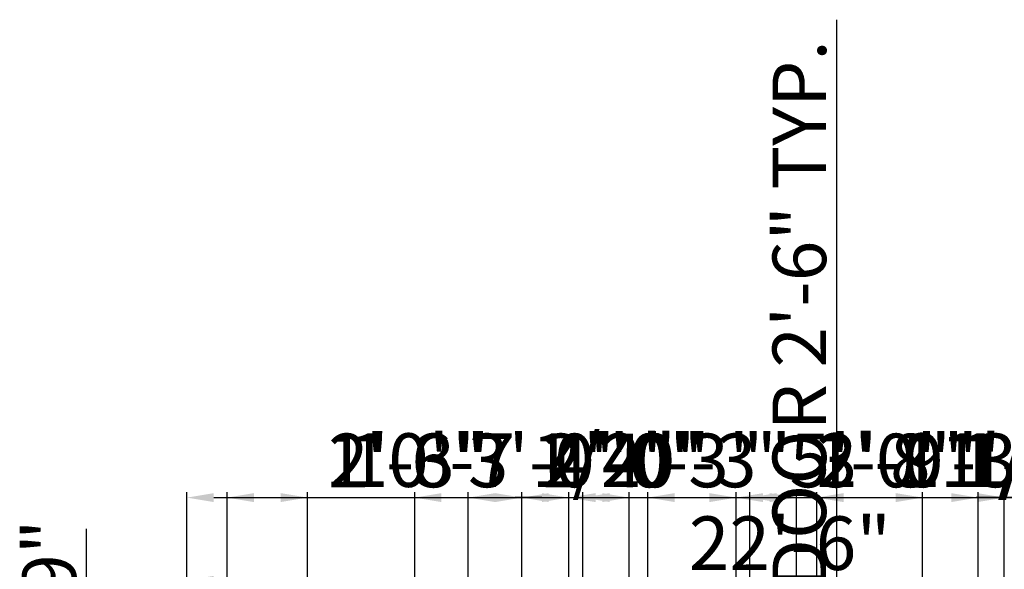
# Model space of a CAD drawing. Units: inches. Extents: x 1086 to 1501, y 383 to 973.
# Tile 6 of 7: x 1096 to 1316, y 850 to 973. Entities that reach past the tile are written whole.
import ezdxf

# ---------------------------------------------------------------- set-up
doc = ezdxf.new("R2010")
doc.units = ezdxf.units.IN
doc.layers.add('A-ANNO-DIMS', color=2, linetype='Continuous', lineweight=18)
doc.styles.get("Standard").update_dxf_attribs({"font": 'arial.ttf'})
doc.dimstyles.new('ISO-25', dxfattribs={"dimtxt": 12, "dimasz": 6, "dimexe": 1.25, "dimexo": 0.625, "dimtad": 1, "dimdec": 1, "dimlunit": 3, "dimtxsty": 'Standard', "dimcen": 2.5, "dimadec": 0, "dimazin": 0, "dimtfac": 1, "dimtdec": 1, "dimtmove": 0, "dimatfit": 3, "dimfxl": 1, "dimarcsym": 0})

# ---------------------------------------------------------------- blocks, each defined once
blk = doc.blocks.new('*D9')
at = {"layer": 'A-ANNO-DIMS', "color": 0, "lineweight": -2, "transparency": 16777216}
for p, q in [((1133.43, 835.83), (1133.43, 848.67)), ((1403.43, 835.83), (1403.43, 848.67)), ((1139.43, 847.42), (1397.43, 847.42))]:
    blk.add_line(p, q, dxfattribs=at)
at = {"layer": 'A-ANNO-DIMS', "color": 0, "transparency": 16777216}
for points in [[(1139.43, 848.42), (1139.43, 846.42), (1133.43, 847.42)], [(1397.43, 848.42), (1397.43, 846.42), (1403.43, 847.42)]]:
    blk.add_solid(points, dxfattribs=at)
at = {"layer": 'Defpoints', "color": 0, "transparency": 16777216}
for p in [(1403.43, 847.42), (1133.43, 835.21), (1403.43, 835.21)]:
    blk.add_point(p, dxfattribs=at)
at = {"layer": 'A-ANNO-DIMS', "color": 0, "transparency": 16777216, "insert": (1268.43, 854.18), "char_height": 12, "attachment_point": 5}
blk.add_mtext('22\'-6"', dxfattribs=at)
blk = doc.blocks.new('*D17')
at = {"layer": 'A-ANNO-DIMS', "color": 0, "lineweight": -2, "transparency": 16777216}
for p, q in [((1278.93, 788.71), (1278.93, 972.89)), ((1275.05, 788.71), (1280.18, 788.71)), ((1278.93, 764.71), (1278.93, 782.71)), ((1275.05, 758.71), (1280.18, 758.71))]:
    blk.add_line(p, q, dxfattribs=at)
at = {"layer": 'A-ANNO-DIMS', "color": 0, "transparency": 16777216}
for points in [[(1277.93, 782.71), (1279.93, 782.71), (1278.93, 788.71)], [(1277.93, 764.71), (1279.93, 764.71), (1278.93, 758.71)]]:
    blk.add_solid(points, dxfattribs=at)
at = {"layer": 'Defpoints', "color": 0, "transparency": 16777216}
for p in [(1274.43, 788.71), (1278.93, 788.71), (1274.43, 758.71)]:
    blk.add_point(p, dxfattribs=at)
at = {"layer": 'A-ANNO-DIMS', "color": 0, "transparency": 16777216, "insert": (1272.1, 883.8), "char_height": 12, "attachment_point": 5, "rotation": 90}
blk.add_mtext('BATH DOOR 2\'-6" TYP.', dxfattribs=at)
blk = doc.blocks.new('*D29')
at = {"layer": 'A-ANNO-DIMS', "color": 0, "lineweight": -2, "transparency": 16777216}
for p, q in [((1133.43, 835.83), (1133.43, 867.19)), ((1160.43, 835.83), (1160.43, 867.19)), ((1139.43, 865.94), (1154.43, 865.94)), ((1160.43, 865.94), (1199.78, 865.94))]:
    blk.add_line(p, q, dxfattribs=at)
at = {"layer": 'A-ANNO-DIMS', "color": 0, "transparency": 16777216}
for points in [[(1139.43, 866.94), (1139.43, 864.94), (1133.43, 865.94)], [(1154.43, 866.94), (1154.43, 864.94), (1160.43, 865.94)]]:
    blk.add_solid(points, dxfattribs=at)
at = {"layer": 'Defpoints', "color": 0, "transparency": 16777216}
for p in [(1160.43, 865.94), (1133.43, 835.21), (1160.43, 835.21)]:
    blk.add_point(p, dxfattribs=at)
at = {"layer": 'A-ANNO-DIMS', "color": 0, "transparency": 16777216, "insert": (1183.11, 872.7), "char_height": 12, "attachment_point": 5}
blk.add_mtext('2\'-3"', dxfattribs=at)
blk = doc.blocks.new('*D30')
at = {"layer": 'A-ANNO-DIMS', "color": 0, "lineweight": -2, "transparency": 16777216}
for p, q in [((1196.43, 835.83), (1196.43, 867.19)), ((1232.43, 835.83), (1232.43, 867.19)), ((1202.43, 865.94), (1226.43, 865.94))]:
    blk.add_line(p, q, dxfattribs=at)
at = {"layer": 'A-ANNO-DIMS', "color": 0, "transparency": 16777216}
for points in [[(1202.43, 866.94), (1202.43, 864.94), (1196.43, 865.94)], [(1226.43, 866.94), (1226.43, 864.94), (1232.43, 865.94)]]:
    blk.add_solid(points, dxfattribs=at)
at = {"layer": 'Defpoints', "color": 0, "transparency": 16777216}
for p in [(1232.43, 865.94), (1196.43, 835.21), (1232.43, 835.21)]:
    blk.add_point(p, dxfattribs=at)
at = {"layer": 'A-ANNO-DIMS', "color": 0, "transparency": 16777216, "insert": (1214.43, 872.7), "char_height": 12, "attachment_point": 5}
blk.add_mtext('3\'-0"', dxfattribs=at)
blk = doc.blocks.new('*D31')
at = {"layer": 'A-ANNO-DIMS', "color": 0, "lineweight": -2, "transparency": 16777216}
for p, q in [((1256.43, 835.83), (1256.43, 867.19)), ((1316.43, 835.83), (1316.43, 867.19)), ((1262.43, 865.94), (1310.43, 865.94))]:
    blk.add_line(p, q, dxfattribs=at)
at = {"layer": 'A-ANNO-DIMS', "color": 0, "transparency": 16777216}
for points in [[(1262.43, 866.94), (1262.43, 864.94), (1256.43, 865.94)], [(1310.43, 866.94), (1310.43, 864.94), (1316.43, 865.94)]]:
    blk.add_solid(points, dxfattribs=at)
at = {"layer": 'Defpoints', "color": 0, "transparency": 16777216}
for p in [(1316.43, 865.94), (1256.43, 835.21), (1316.43, 835.21)]:
    blk.add_point(p, dxfattribs=at)
at = {"layer": 'A-ANNO-DIMS', "color": 0, "transparency": 16777216, "insert": (1286.43, 872.69), "char_height": 12, "attachment_point": 5}
blk.add_mtext('5\'-0"', dxfattribs=at)
blk = doc.blocks.new('*D40')
at = {"layer": 'A-ANNO-DIMS', "color": 0, "lineweight": -2, "transparency": 16777216}
for p, q in [((1142.43, 502.33), (1142.43, 867.19)), ((1269.93, 502.33), (1269.93, 867.19)), ((1148.43, 865.94), (1263.93, 865.94))]:
    blk.add_line(p, q, dxfattribs=at)
at = {"layer": 'A-ANNO-DIMS', "color": 0, "transparency": 16777216}
for points in [[(1148.43, 866.94), (1148.43, 864.94), (1142.43, 865.94)], [(1263.93, 866.94), (1263.93, 864.94), (1269.93, 865.94)]]:
    blk.add_solid(points, dxfattribs=at)
at = {"layer": 'Defpoints', "color": 0, "transparency": 16777216}
for p in [(1269.93, 865.94), (1142.43, 501.71), (1269.93, 501.71)]:
    blk.add_point(p, dxfattribs=at)
at = {"layer": 'A-ANNO-DIMS', "color": 0, "transparency": 16777216, "insert": (1206.18, 872.77), "char_height": 12, "attachment_point": 5}
blk.add_mtext('10\'-7 1/2"', dxfattribs=at)
blk = doc.blocks.new('*D42')
at = {"layer": 'A-ANNO-DIMS', "color": 0, "lineweight": -2, "transparency": 16777216}
for p, q in [((1256.43, 502.33), (1256.43, 867.19)), ((1269.93, 502.33), (1269.93, 867.19)), ((1262.43, 865.94), (1263.93, 865.94)), ((1269.93, 865.94), (1335.91, 865.94))]:
    blk.add_line(p, q, dxfattribs=at)
at = {"layer": 'A-ANNO-DIMS', "color": 0, "transparency": 16777216}
for points in [[(1262.43, 866.94), (1262.43, 864.94), (1256.43, 865.94)], [(1263.93, 866.94), (1263.93, 864.94), (1269.93, 865.94)]]:
    blk.add_solid(points, dxfattribs=at)
at = {"layer": 'Defpoints', "color": 0, "transparency": 16777216}
for p in [(1269.93, 865.94), (1256.43, 501.71), (1269.93, 501.71)]:
    blk.add_point(p, dxfattribs=at)
at = {"layer": 'A-ANNO-DIMS', "color": 0, "transparency": 16777216, "insert": (1305.92, 872.77), "char_height": 12, "attachment_point": 5}
blk.add_mtext('1\'-1 1/2"', dxfattribs=at)
blk = doc.blocks.new('*D43')
at = {"layer": 'A-ANNO-DIMS', "color": 0, "lineweight": -2, "transparency": 16777216}
for p, q in [((1208.43, 497.83), (1208.43, 867.19)), ((1256.43, 497.83), (1256.43, 867.19)), ((1214.43, 865.94), (1250.43, 865.94))]:
    blk.add_line(p, q, dxfattribs=at)
at = {"layer": 'A-ANNO-DIMS', "color": 0, "transparency": 16777216}
for points in [[(1214.43, 866.94), (1214.43, 864.94), (1208.43, 865.94)], [(1250.43, 866.94), (1250.43, 864.94), (1256.43, 865.94)]]:
    blk.add_solid(points, dxfattribs=at)
at = {"layer": 'Defpoints', "color": 0, "transparency": 16777216}
for p in [(1256.43, 865.94), (1208.43, 497.21), (1256.43, 497.21)]:
    blk.add_point(p, dxfattribs=at)
at = {"layer": 'A-ANNO-DIMS', "color": 0, "transparency": 16777216, "insert": (1232.43, 872.69), "char_height": 12, "attachment_point": 5}
blk.add_mtext('4\'-0"', dxfattribs=at)
blk = doc.blocks.new('*D45')
at = {"layer": 'A-ANNO-DIMS', "color": 0, "lineweight": -2, "transparency": 16777216}
for p, q in [((1259.43, 497.83), (1259.43, 867.19)), ((1358.43, 497.83), (1358.43, 867.19)), ((1265.43, 865.94), (1352.43, 865.94))]:
    blk.add_line(p, q, dxfattribs=at)
at = {"layer": 'A-ANNO-DIMS', "color": 0, "transparency": 16777216}
for points in [[(1265.43, 866.94), (1265.43, 864.94), (1259.43, 865.94)], [(1352.43, 866.94), (1352.43, 864.94), (1358.43, 865.94)]]:
    blk.add_solid(points, dxfattribs=at)
at = {"layer": 'Defpoints', "color": 0, "transparency": 16777216}
for p in [(1358.43, 865.94), (1259.43, 497.21), (1358.43, 497.21)]:
    blk.add_point(p, dxfattribs=at)
at = {"layer": 'A-ANNO-DIMS', "color": 0, "transparency": 16777216, "insert": (1308.93, 872.7), "char_height": 12, "attachment_point": 5}
blk.add_mtext('8\'-3"', dxfattribs=at)
blk = doc.blocks.new('*D50')
at = {"layer": 'A-ANNO-DIMS', "color": 0, "lineweight": -2, "transparency": 16777216}
for p, q in [((1184.43, 502.33), (1184.43, 867.19)), ((1208.43, 502.33), (1208.43, 867.19)), ((1190.43, 865.94), (1202.43, 865.94)), ((1208.43, 865.94), (1247.78, 865.94))]:
    blk.add_line(p, q, dxfattribs=at)
at = {"layer": 'A-ANNO-DIMS', "color": 0, "transparency": 16777216}
for points in [[(1190.43, 866.94), (1190.43, 864.94), (1184.43, 865.94)], [(1202.43, 866.94), (1202.43, 864.94), (1208.43, 865.94)]]:
    blk.add_solid(points, dxfattribs=at)
at = {"layer": 'Defpoints', "color": 0, "transparency": 16777216}
for p in [(1208.43, 865.94), (1184.43, 501.71), (1208.43, 501.71)]:
    blk.add_point(p, dxfattribs=at)
at = {"layer": 'A-ANNO-DIMS', "color": 0, "transparency": 16777216, "insert": (1231.11, 872.69), "char_height": 12, "attachment_point": 5}
blk.add_mtext('2\'-0"', dxfattribs=at)
blk = doc.blocks.new('*D55')
at = {"layer": 'A-ANNO-DIMS', "color": 0, "lineweight": -2, "transparency": 16777216}
for p, q in [((1218.93, 826.83), (1218.93, 867.19)), ((1222.08, 821.57), (1222.08, 867.19)), ((1212.93, 865.94), (1206.93, 865.94)), ((1218.93, 865.94), (1222.08, 865.94)), ((1228.08, 865.94), (1267.23, 865.94))]:
    blk.add_line(p, q, dxfattribs=at)
at = {"layer": 'A-ANNO-DIMS', "color": 0, "transparency": 16777216}
for points in [[(1212.93, 866.94), (1212.93, 864.94), (1218.93, 865.94)], [(1228.08, 866.94), (1228.08, 864.94), (1222.08, 865.94)]]:
    blk.add_solid(points, dxfattribs=at)
at = {"layer": 'Defpoints', "color": 0, "transparency": 16777216}
for p in [(1222.08, 865.94), (1218.93, 826.21), (1222.08, 820.94)]:
    blk.add_point(p, dxfattribs=at)
at = {"layer": 'A-ANNO-DIMS', "color": 0, "transparency": 16777216, "insert": (1250.66, 872.7), "char_height": 12, "attachment_point": 5}
blk.add_mtext('0\'-3"', dxfattribs=at)
blk = doc.blocks.new('*D57')
at = {"layer": 'A-ANNO-DIMS', "color": 0, "lineweight": -2, "transparency": 16777216}
for p, q in [((1110.93, 820.94), (1110.93, 858.96)), ((1221.46, 820.94), (1109.68, 820.94)), ((1110.93, 805.94), (1110.93, 814.94)), ((1221.46, 799.94), (1109.68, 799.94))]:
    blk.add_line(p, q, dxfattribs=at)
at = {"layer": 'A-ANNO-DIMS', "color": 0, "transparency": 16777216}
for points in [[(1109.93, 814.94), (1111.93, 814.94), (1110.93, 820.94)], [(1109.93, 805.94), (1111.93, 805.94), (1110.93, 799.94)]]:
    blk.add_solid(points, dxfattribs=at)
at = {"layer": 'Defpoints', "color": 0, "transparency": 16777216}
for p in [(1110.93, 820.94), (1222.08, 820.94), (1222.08, 799.94)]:
    blk.add_point(p, dxfattribs=at)
at = {"layer": 'A-ANNO-DIMS', "color": 0, "transparency": 16777216, "insert": (1104.18, 842.95), "char_height": 12, "attachment_point": 5, "rotation": 90}
blk.add_mtext('1\'-9"', dxfattribs=at)
blk = doc.blocks.new('*D59')
at = {"layer": 'A-ANNO-DIMS', "color": 0, "lineweight": -2, "transparency": 16777216}
for p, q in [((1218.93, 826.83), (1218.93, 867.19)), ((1269.93, 826.83), (1269.93, 867.19)), ((1224.93, 865.94), (1263.93, 865.94))]:
    blk.add_line(p, q, dxfattribs=at)
at = {"layer": 'A-ANNO-DIMS', "color": 0, "transparency": 16777216}
for points in [[(1224.93, 866.94), (1224.93, 864.94), (1218.93, 865.94)], [(1263.93, 866.94), (1263.93, 864.94), (1269.93, 865.94)]]:
    blk.add_solid(points, dxfattribs=at)
at = {"layer": 'Defpoints', "color": 0, "transparency": 16777216}
for p in [(1269.93, 865.94), (1218.93, 826.21), (1269.93, 826.21)]:
    blk.add_point(p, dxfattribs=at)
at = {"layer": 'A-ANNO-DIMS', "color": 0, "transparency": 16777216, "insert": (1244.43, 872.7), "char_height": 12, "attachment_point": 5}
blk.add_mtext('4\'-3"', dxfattribs=at)
blk = doc.blocks.new('*D61')
at = {"layer": 'A-ANNO-DIMS', "color": 0, "lineweight": -2, "transparency": 16777216}
for p, q in [((1382.11, 674.69), (1382.11, 867.19)), ((1394.43, 678.33), (1394.43, 867.19)), ((1376.11, 865.94), (1310.13, 865.94)), ((1394.43, 865.94), (1382.11, 865.94)), ((1400.43, 865.94), (1406.43, 865.94))]:
    blk.add_line(p, q, dxfattribs=at)
at = {"layer": 'A-ANNO-DIMS', "color": 0, "transparency": 16777216}
for points in [[(1376.11, 866.94), (1376.11, 864.94), (1382.11, 865.94)], [(1400.43, 866.94), (1400.43, 864.94), (1394.43, 865.94)]]:
    blk.add_solid(points, dxfattribs=at)
at = {"layer": 'Defpoints', "color": 0, "transparency": 16777216}
for p in [(1382.11, 865.94), (1394.43, 677.71), (1382.11, 674.06)]:
    blk.add_point(p, dxfattribs=at)
at = {"layer": 'A-ANNO-DIMS', "color": 0, "transparency": 16777216, "insert": (1340.12, 872.77), "char_height": 12, "attachment_point": 5}
blk.add_mtext('1\'-0 1/2"', dxfattribs=at)
blk = doc.blocks.new('*D69')
at = {"layer": 'A-ANNO-DIMS', "color": 0, "lineweight": -2, "transparency": 16777216}
for p, q in [((1236.63, 603.21), (1236.63, 867.19)), ((1269.93, 603.25), (1269.93, 867.19)), ((1242.63, 865.94), (1263.93, 865.94)), ((1269.93, 865.94), (1337.25, 865.94))]:
    blk.add_line(p, q, dxfattribs=at)
at = {"layer": 'A-ANNO-DIMS', "color": 0, "transparency": 16777216}
for points in [[(1242.63, 866.94), (1242.63, 864.94), (1236.63, 865.94)], [(1263.93, 866.94), (1263.93, 864.94), (1269.93, 865.94)]]:
    blk.add_solid(points, dxfattribs=at)
at = {"layer": 'Defpoints', "color": 0, "transparency": 16777216}
for p in [(1269.93, 865.94), (1236.63, 602.59), (1269.93, 602.62)]:
    blk.add_point(p, dxfattribs=at)
at = {"layer": 'A-ANNO-DIMS', "color": 0, "transparency": 16777216, "insert": (1306.59, 872.77), "char_height": 12, "attachment_point": 5}
blk.add_mtext('2\'-9 1/2"', dxfattribs=at)
blk = doc.blocks.new('*D71')
at = {"layer": 'A-ANNO-DIMS', "color": 0, "lineweight": -2, "transparency": 16777216}
for p, q in [((1142.43, 589.29), (1142.43, 867.19)), ((1160.43, 589.29), (1160.43, 867.19)), ((1148.43, 865.94), (1154.43, 865.94)), ((1160.43, 865.94), (1198.45, 865.94))]:
    blk.add_line(p, q, dxfattribs=at)
at = {"layer": 'A-ANNO-DIMS', "color": 0, "transparency": 16777216}
for points in [[(1148.43, 866.94), (1148.43, 864.94), (1142.43, 865.94)], [(1154.43, 866.94), (1154.43, 864.94), (1160.43, 865.94)]]:
    blk.add_solid(points, dxfattribs=at)
at = {"layer": 'Defpoints', "color": 0, "transparency": 16777216}
for p in [(1160.43, 865.94), (1142.43, 588.67), (1160.43, 588.67)]:
    blk.add_point(p, dxfattribs=at)
at = {"layer": 'A-ANNO-DIMS', "color": 0, "transparency": 16777216, "insert": (1182.44, 872.69), "char_height": 12, "attachment_point": 5}
blk.add_mtext('1\'-6"', dxfattribs=at)
blk = doc.blocks.new('*D75')
at = {"layer": 'A-ANNO-DIMS', "color": 0, "lineweight": -2, "transparency": 16777216}
for p, q in [((1274.43, 723.33), (1274.43, 867.19)), ((1310.55, 724.51), (1310.55, 867.19)), ((1280.43, 865.94), (1304.55, 865.94))]:
    blk.add_line(p, q, dxfattribs=at)
at = {"layer": 'A-ANNO-DIMS', "color": 0, "transparency": 16777216}
for points in [[(1280.43, 866.94), (1280.43, 864.94), (1274.43, 865.94)], [(1304.55, 866.94), (1304.55, 864.94), (1310.55, 865.94)]]:
    blk.add_solid(points, dxfattribs=at)
at = {"layer": 'Defpoints', "color": 0, "transparency": 16777216}
for p in [(1310.55, 865.94), (1310.55, 723.89), (1274.43, 722.71)]:
    blk.add_point(p, dxfattribs=at)
at = {"layer": 'A-ANNO-DIMS', "color": 0, "transparency": 16777216, "insert": (1292.49, 872.7), "char_height": 12, "attachment_point": 5}
blk.add_mtext('3\'-0"', dxfattribs=at)
blk = doc.blocks.new('*D77')
at = {"layer": 'A-ANNO-DIMS', "color": 0, "lineweight": -2, "transparency": 16777216}
for p, q in [((1274.43, 502.33), (1274.43, 867.19)), ((1298.14, 513.04), (1298.14, 867.19)), ((1280.43, 865.94), (1292.14, 865.94)), ((1298.14, 865.94), (1373.44, 865.94))]:
    blk.add_line(p, q, dxfattribs=at)
at = {"layer": 'A-ANNO-DIMS', "color": 0, "transparency": 16777216}
for points in [[(1280.43, 866.94), (1280.43, 864.94), (1274.43, 865.94)], [(1292.14, 866.94), (1292.14, 864.94), (1298.14, 865.94)]]:
    blk.add_solid(points, dxfattribs=at)
at = {"layer": 'Defpoints', "color": 0, "transparency": 16777216}
for p in [(1298.14, 865.94), (1298.14, 512.42), (1274.43, 501.71)]:
    blk.add_point(p, dxfattribs=at)
at = {"layer": 'A-ANNO-DIMS', "color": 0, "transparency": 16777216, "insert": (1338.79, 872.77), "char_height": 12, "attachment_point": 5}
blk.add_mtext('1\'-11 1/2"', dxfattribs=at)

msp = doc.modelspace()

# ---------------------------------------------------------------- dimensions: what is measured, and where the dimension line sits
at = {"layer": 'A-ANNO-DIMS'}
dim = msp.add_linear_dim(base=(1278.93, 788.71), p1=(1274.43, 758.71), p2=(1274.43, 788.71), angle=90, text='BATH DOOR <> TYP.', dimstyle='ISO-25', override={"dimdec": 1, "dimlfac": 1, "dimrnd": 0, "dimzin": 1, "dimdsep": 46, "dimlunit": 4, "dimfrac": 2}, dxfattribs=at)
dim.commit()
dim.dimension.update_dxf_attribs({"geometry": '*D17', "text_midpoint": (1272.1, 883.8)})
for base, p1, p2, override, picture, middle in [((1269.93, 865.94), (1142.43, 501.71), (1269.93, 501.71), {"dimdec": 1, "dimlfac": 1, "dimrnd": 0, "dimzin": 1, "dimdsep": 46, "dimlunit": 4, "dimfrac": 2}, '*D40', (1206.18, 872.77)), ((1269.93, 865.94), (1236.63, 602.59), (1269.93, 602.62), {"dimdec": 1, "dimlfac": 1, "dimrnd": 0, "dimzin": 1, "dimdsep": 46, "dimlunit": 4, "dimfrac": 2}, '*D69', (1306.59, 872.77)), ((1269.93, 865.94), (1256.43, 501.71), (1269.93, 501.71), {"dimdec": 1, "dimlfac": 1, "dimrnd": 0, "dimzin": 1, "dimdsep": 46, "dimlunit": 4, "dimfrac": 2}, '*D42', (1305.92, 872.77)), ((1298.14, 865.94), (1274.43, 501.71), (1298.14, 512.42), {"dimdec": 1, "dimlfac": 1, "dimrnd": 0, "dimzin": 1, "dimdsep": 46, "dimlunit": 4, "dimfrac": 2}, '*D77', (1338.79, 872.77)), ((1382.11, 865.94), (1394.43, 677.71), (1382.11, 674.06), {"dimdec": 1, "dimlfac": 1, "dimrnd": 0, "dimzin": 1, "dimdsep": 46, "dimlunit": 4, "dimfrac": 2}, '*D61', (1340.12, 872.77)), ((1160.43, 865.94), (1133.43, 835.21), (1160.43, 835.21), {"dimdec": 1, "dimlfac": 1, "dimrnd": 0, "dimzin": 1, "dimdsep": 46, "dimlunit": 4, "dimfrac": 2}, '*D29', (1183.11, 872.7)), ((1160.43, 865.94), (1142.43, 588.67), (1160.43, 588.67), {"dimdec": 1, "dimlfac": 1, "dimrnd": 0, "dimzin": 1, "dimdsep": 46, "dimlunit": 4, "dimfrac": 2}, '*D71', (1182.44, 872.69)), ((1208.43, 865.94), (1184.43, 501.71), (1208.43, 501.71), {"dimdec": 1, "dimlfac": 1, "dimrnd": 0, "dimzin": 1, "dimdsep": 46, "dimlunit": 4, "dimfrac": 2}, '*D50', (1231.11, 872.69)), ((1232.43, 865.94), (1196.43, 835.21), (1232.43, 835.21), {"dimdec": 1, "dimlfac": 1, "dimrnd": 0, "dimzin": 1, "dimdsep": 46, "dimlunit": 4, "dimfrac": 2}, '*D30', (1214.43, 872.7)), ((1222.0839, 865.9409), (1218.9297, 826.2068), (1222.0839, 820.9409), {"dimdec": 1, "dimlfac": 1, "dimrnd": 0, "dimzin": 1, "dimdsep": 46, "dimlunit": 4, "dimfrac": 2}, '*D55', (1250.6584, 872.6968)), ((1256.43, 865.94), (1208.43, 497.21), (1256.43, 497.21), {"dimdec": 1, "dimlfac": 1, "dimrnd": 0, "dimzin": 1, "dimdsep": 46, "dimlunit": 4, "dimfrac": 2}, '*D43', (1232.43, 872.69)), ((1269.93, 865.94), (1218.93, 826.21), (1269.93, 826.21), {"dimdec": 1, "dimlfac": 1, "dimrnd": 0, "dimzin": 1, "dimdsep": 46, "dimlunit": 4, "dimfrac": 2}, '*D59', (1244.43, 872.7)), ((1316.43, 865.94), (1256.43, 835.21), (1316.43, 835.21), {"dimdec": 1, "dimlfac": 1, "dimrnd": 0, "dimzin": 1, "dimdsep": 46, "dimlunit": 4, "dimfrac": 2}, '*D31', (1286.43, 872.69)), ((1358.43, 865.94), (1259.43, 497.21), (1358.43, 497.21), {"dimdec": 1, "dimlfac": 1, "dimrnd": 0, "dimzin": 1, "dimdsep": 46, "dimlunit": 4, "dimfrac": 2}, '*D45', (1308.93, 872.7)), ((1310.55, 865.94), (1274.43, 722.71), (1310.55, 723.89), {"dimdec": 1, "dimlfac": 1, "dimrnd": 0, "dimzin": 1, "dimdsep": 46, "dimlunit": 4, "dimfrac": 2}, '*D75', (1292.49, 872.7)), ((1403.43, 847.42), (1133.43, 835.21), (1403.43, 835.21), {"dimclrd": 0, "dimclre": 0, "dimclrt": 0}, '*D9', (1268.43, 854.18))]:
    dim = msp.add_linear_dim(base=base, p1=p1, p2=p2, dimstyle='ISO-25', override=override, dxfattribs=at)
    dim.commit()
    dim.dimension.update_dxf_attribs({"geometry": picture, "text_midpoint": middle})
dim = msp.add_linear_dim(base=(1110.93, 820.94), p1=(1222.08, 799.94), p2=(1222.08, 820.94), angle=90, dimstyle='ISO-25', override={"dimdec": 1, "dimlfac": 1, "dimrnd": 0, "dimzin": 1, "dimdsep": 46, "dimlunit": 4, "dimfrac": 2}, dxfattribs=at)
dim.commit()
dim.dimension.update_dxf_attribs({"geometry": '*D57', "text_midpoint": (1104.18, 842.95)})

doc.saveas('drawing.dxf')
